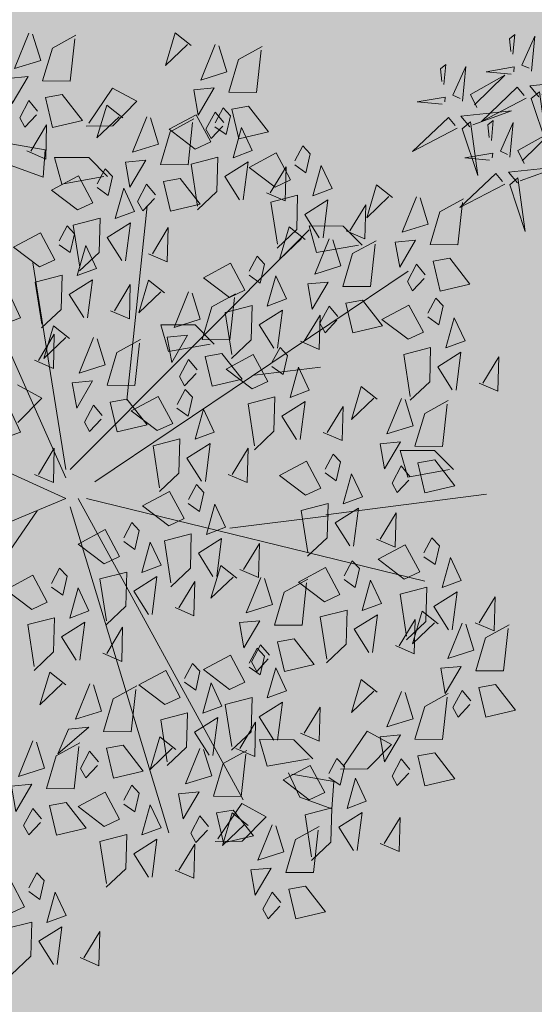
# Model space of a CAD drawing. Units: inches. Extents: x 1704 to 6393, y -157 to 1172.
# Tile 68 of 122: x 1913 to 1928, y 980 to 1010. Entities that reach past the tile are written whole.
import ezdxf

# ---------------------------------------------------------------- set-up
doc = ezdxf.new("R2010")
doc.units = ezdxf.units.IN
doc.header["$MEASUREMENT"] = 0
for name, color, linetype, lineweight in [('A-ANNO-DIMS', 7, 'Continuous', 13), ('L-shrub', 74, 'Continuous', 18), ('L-tree', 102, 'Continuous', 18)]:
    doc.layers.add(name, color=color, linetype=linetype, lineweight=lineweight)
doc.layers.add('L-HRDS-PATT', color=9, linetype='Continuous', lineweight=13, true_color=0xc5c1ba)
doc.styles.get("Standard").update_dxf_attribs({"font": 'arial.ttf'})
doc.dimstyles.get("Standard").update_dxf_attribs({"dimtxt": 6, "dimasz": 2, "dimexe": 0.18, "dimexo": 0.0625, "dimgap": 0.09, "dimtad": 0, "dimtih": 1, "dimtoh": 1, "dimdec": 1, "dimzin": 0, "dimdsep": 46, "dimlunit": 3, "dimtxsty": 'Standard', "dimblk": 'ARCHTICK', "dimcen": 0.09, "dimadec": 0, "dimazin": 0, "dimtfac": 1, "dimtdec": 1, "dimtofl": 0, "dimtmove": 0, "dimatfit": 3, "dimfxl": 1, "dimtolj": 1, "dimtzin": 0, "dimarcsym": 0})

# ---------------------------------------------------------------- blocks, each defined once
blk = doc.blocks.new('bamboo')
at = {"layer": 'L-shrub'}
for points in [[(1141.3, 824.7), (1092, 972.3), (1115.5, 803.4), (1141.3, 824.7)], [(1157.1, 823.2), (1299, 896.7), (1185.5, 788.7), (1164.2, 814.6)], [(1117, 819.1), (1145.4, 784.6), (985.2, 768.4), (1108.4, 812)], [(1291.5, 647.4), (1242.1, 795), (1265.7, 626.1), (1291.5, 647.4)], [(1095.3, 757.7), (1115.1, 716.2), (1006.1, 655.3), (1102.4, 749.1)], [(1140.9, 737.5), (1130.4, 627.4), (1170.9, 718.7), (1148, 728.8)], [(1205.3, 747.1), (1283.9, 739.5), (1195.2, 724.3), (1196.7, 740)], [(1307.2, 645.9), (1449.1, 719.5), (1335.7, 611.4), (1314.3, 637.3)], [(1073.1, 552), (1023.7, 699.6), (1047.2, 530.7), (1073.1, 552)], [(1199.3, 684.2), (1193.3, 621.3), (1210.5, 635.5), (1206.4, 675.6)], [(1088.8, 550.5), (1230.7, 624), (1117.2, 516), (1095.9, 541.8)], [(1267.2, 641.9), (1295.6, 607.4), (1135.4, 591.1), (1258.6, 634.8)], [(1245.4, 580.5), (1265.3, 538.9), (1156.3, 478), (1252.6, 571.9)], [(1355.5, 569.8), (1434.1, 562.2), (1345.4, 547), (1346.9, 562.7)], [(1048.7, 546.4), (1077.2, 511.9), (916.9, 495.7), (1040.1, 539.3)], [(1291.1, 560.2), (1280.6, 450.1), (1321.1, 541.4), (1298.2, 551.6)], [(1349.5, 506.9), (1343.5, 444), (1360.7, 458.2), (1356.6, 498.3)], [(1137.1, 474.4), (1215.7, 466.8), (1126.9, 451.6), (1128.4, 467.3)], [(1072.7, 464.7), (1062.1, 354.7), (1102.6, 446), (1079.8, 456.1)], [(1131.1, 411.5), (1125, 348.6), (1142.3, 362.8), (1138.2, 402.9)]]:
    blk.add_lwpolyline(points, dxfattribs=at)
blk = doc.blocks.new('flower shrub 3')
at = {"layer": 'L-shrub'}
for p, q in [((208.75, 44.35), (204.49, 19.45)), ((57.01, 21.38), (42.5, 35.62)), ((64.85, 35.82), (57.01, 21.38)), ((188.1, 20.61), (195.06, 39.71)), ((204.49, 19.45), (188.1, 20.61)), ((184.09, 9.47), (199.9, 13.93)), ((199.9, 13.93), (199.81, -6.4)), ((188.5, -15.39), (184.09, 9.47)), ((218.7, -20.78), (218.53, -4.82)), ((199.81, -6.4), (188.49, -17.65)), ((220.15, -6.4), (241.04, -20.58)), ((233.21, -35.02), (218.7, -20.78)), ((241.04, -20.58), (233.21, -35.02)), ((84.69, -53.7), (100.5, -49.25)), ((100.5, -49.25), (100.42, -69.58)), ((89.1, -78.57), (84.69, -53.7)), ((100.42, -69.58), (89.1, -80.83)), ((-205.99, -97.49), (-206.15, -81.53)), ((-204.54, -83.11), (-183.64, -97.29)), ((-191.47, -111.73), (-205.99, -97.49)), ((-183.64, -97.29), (-191.47, -111.73)), ((-161.53, -112.36), (-145.72, -107.91)), ((-145.72, -107.91), (-145.8, -128.24)), ((-157.12, -137.23), (-161.53, -112.36)), ((-179.93, -131.75), (-165.46, -125)), ((-166.23, -127.12), (-170.5, -152.01)), ((-145.8, -128.24), (-157.13, -139.49)), ((-186.88, -150.86), (-179.93, -131.75)), ((143.42, -141.69), (159.24, -137.24)), ((159.24, -137.24), (159.15, -157.57)), ((147.84, -166.56), (143.42, -141.69)), ((-170.5, -152.01), (-186.88, -150.86)), ((-163.07, -171.95), (-163.23, -155.98)), ((-161.62, -157.57), (-140.72, -171.75)), ((159.15, -157.57), (147.83, -168.82)), ((-148.55, -186.18), (-163.07, -171.95)), ((-140.72, -171.75), (-148.55, -186.18)), ((10.15, -195.84), (25.96, -191.38)), ((25.96, -191.38), (25.88, -211.71)), ((14.56, -220.7), (10.15, -195.84)), ((25.88, -211.71), (14.55, -222.96))]:
    blk.add_line(p, q, dxfattribs=at)
for points in [[(-2.54, 7.13), (56.31, 136.92)], [(-9.89, 24.27), (-166.82, 132.02)], [(-2.54, 7.13), (-51.58, 124.68)], [(9.72, 7.13), (124.97, 58.56)], [(-249.17, 40.85), (-237.45, 56.33), (-228.85, 40.3), (-244.9, 31.7), (-249.17, 40.85)], [(-283.1, 39.51), (-258.14, 43.35), (-254.05, 27.44), (-274.37, 27.98), (-285.36, 39.57)], [(-68.45, 27.31), (-56.74, 42.79), (-48.13, 26.76), (-64.18, 18.17), (-68.45, 27.31)], [(32.59, 45.49), (36.8, 34.09), (50.54, 40.49), (32.59, 45.49)], [(100.36, 45.49), (104.57, 34.09), (118.3, 40.49), (100.36, 45.49)], [(247.89, 29.6), (246.76, 41.7), (231.84, 39.06), (247.89, 29.6)], [(-172.27, 27.35), (-173.4, 39.44), (-188.32, 36.8), (-172.27, 27.35)], [(-147.16, 24.62), (-162.72, 19.81), (-167.54, 35.36), (-146.52, 26.78)], [(134.85, 22.8), (146.57, 38.28), (155.17, 22.25), (139.12, 13.65), (134.85, 22.8)], [(273, 26.88), (257.44, 22.07), (252.62, 37.61), (273.64, 29.04)], [(-192.8, 21.66), (-186.55, 26.86), (-196.74, 32.23), (-202.35, 29.19), (-194.97, 22.3)], [(-102.39, 25.97), (-77.43, 29.81), (-73.34, 13.9), (-93.66, 14.45), (-104.64, 26.03)], [(203.73, 30.25), (198.91, 19.1), (219.23, 18.55), (203.67, 28)], [(227.36, 23.91), (233.62, 29.12), (223.43, 34.49), (217.81, 31.44), (225.2, 24.55)], [(-235.92, 29.2), (-240.62, 22.56), (-229.39, 20), (-224.76, 24.39), (-233.67, 29.14)], [(11.72, 25.74), (6.9, 14.58), (27.22, 14.04), (11.66, 23.48)], [(14.63, 7.13), (137.23, 26.72)], [(79.49, 25.74), (74.67, 14.58), (94.99, 14.04), (79.43, 23.48)], [(100.92, 21.46), (125.88, 25.3), (129.97, 9.39), (109.65, 9.94), (98.66, 21.52)], [(-279.26, 14.57), (-265.46, 23.23), (-256.8, 9.45), (-279.32, 12.32)], [(-254.29, 18.41), (-250.08, 7.02), (-236.35, 13.42), (-254.29, 18.41)], [(-149.87, -0.46), (-174.98, 2.27), (-174.83, 18.69), (-155.34, 12.92), (-147.71, -1.1)], [(-113.13, 7.2), (-105.6, 16.74), (-125.09, 22.51), (-112.49, 9.37)], [(92.43, 4.95), (99.97, 14.48), (80.47, 20.25), (93.07, 7.11)], [(237.16, 9.25), (221.85, -2.69), (217.66, 15.02), (235.39, 19.19), (237.16, 9.25)], [(270.29, 1.8), (245.18, 4.52), (245.33, 20.95), (264.83, 15.18), (272.46, 1.16)], [(-183.01, 6.99), (-198.32, -4.95), (-202.5, 12.76), (-184.78, 16.93), (-183.01, 6.99)], [(-138.39, -6.5), (-139.52, 5.6), (-154.26, 11.88), (-138.39, -6.5)], [(-55.21, 15.67), (-59.91, 9.02), (-48.68, 6.46), (-44.04, 10.85), (-52.95, 15.61)], [(168.74, 0.24), (180.45, 15.72), (189.06, -0.31), (173.01, -8.91), (168.74, 0.24)], [(-98.54, 1.04), (-84.75, 9.69), (-76.08, -4.08), (-98.6, -1.22)], [(148.1, 11.15), (143.4, 4.51), (154.63, 1.95), (159.26, 6.34), (150.35, 11.09)], [(-7.44, 4.68), (-201.15, -54.09)], [(-113.28, -9.22), (-128.84, -14.03), (-133.66, 1.52), (-112.64, -7.06)], [(-73.58, 4.88), (-69.37, -6.52), (-55.64, -0.12), (-73.58, 4.88)], [(14.63, 4.68), (156.84, -137.36)], [(67.18, -8.75), (66.05, 3.35), (51.13, 0.7), (67.18, -8.75)], [(104.77, -3.47), (118.56, 5.18), (127.22, -8.59), (104.7, -5.73)], [(129.73, 0.37), (133.94, -11.03), (147.67, -4.63), (129.73, 0.37)], [(134.8, -1.11), (159.76, 2.73), (163.85, -13.17), (143.53, -12.63), (132.54, -1.04)], [(-275.17, -1.33), (-279.99, -12.49), (-259.66, -13.04), (-275.23, -3.59)], [(-197.21, -15.56), (-185.5, -0.08), (-176.89, -16.11), (-192.94, -24.7), (-197.21, -15.56)], [(-2.54, -0.22), (-181.53, -98.18)], [(-158.92, -12.19), (-152.66, -6.98), (-162.85, -1.61), (-168.47, -4.65), (-161.08, -11.54)], [(-2.54, -5.12), (-51.58, -205.93)], [(-41.35, -15.56), (-29.63, -0.08), (-21.02, -16.11), (-37.07, -24.7), (-41.35, -15.56)], [(46.65, -14.44), (52.9, -9.23), (42.71, -3.87), (37.1, -6.91), (44.48, -13.8)], [(92.28, -11.48), (76.73, -16.28), (71.9, -0.74), (92.92, -9.31)], [(7.27, -10.01), (132.32, -196.13)], [(181.98, -11.41), (177.28, -18.05), (188.51, -20.61), (193.15, -16.22), (184.24, -11.47)], [(223.45, -26.64), (230.99, -17.1), (211.49, -11.33), (224.09, -24.47)], [(-231.15, -16.9), (-206.18, -13.06), (-202.09, -28.97), (-222.42, -28.42), (-233.4, -16.84)], [(-149.12, -26.85), (-164.43, -38.79), (-168.62, -21.08), (-150.89, -16.91), (-149.12, -26.85)], [(-115.99, -34.3), (-141.1, -31.58), (-140.95, -15.15), (-121.45, -20.92), (-113.82, -34.94)], [(-94.45, -14.87), (-99.27, -26.03), (-78.95, -26.58), (-94.51, -17.13)], [(-75.28, -16.9), (-50.32, -13.06), (-46.23, -28.97), (-66.55, -28.42), (-77.54, -16.84)], [(89.57, -36.56), (64.47, -33.83), (64.62, -17.41), (84.11, -23.18), (91.74, -37.2)], [(138.65, -26.04), (152.44, -17.38), (161.11, -31.16), (138.59, -28.29)], [(56.44, -29.1), (41.13, -41.04), (36.95, -23.34), (54.67, -19.17), (56.44, -29.1)], [(108.86, -19.38), (104.03, -30.54), (124.36, -31.09), (108.79, -21.64)], [(163.61, -22.2), (167.82, -33.59), (181.55, -27.19), (163.61, -22.2)], [(-183.97, -27.2), (-188.67, -33.84), (-177.44, -36.4), (-172.8, -32.02), (-181.71, -27.26)], [(-28.1, -27.2), (-32.8, -33.84), (-21.57, -36.4), (-16.93, -32.02), (-25.84, -27.26)], [(55.85, -28.96), (171.09, -41.21)], [(198.2, -40.34), (197.06, -28.24), (182.15, -30.88), (198.2, -40.34)], [(-227.3, -41.83), (-213.51, -33.17), (-204.84, -46.95), (-227.36, -44.08)], [(-71.43, -41.83), (-57.64, -33.17), (-48.97, -46.95), (-71.49, -44.08)], [(37.72, -47.14), (49.43, -31.66), (58.04, -47.69), (41.99, -56.29), (37.72, -47.14)], [(223.3, -43.06), (207.75, -47.87), (202.92, -32.33), (223.94, -40.9)], [(-202.34, -37.99), (-198.13, -49.39), (-184.4, -42.99), (-202.34, -37.99)], [(-124.93, -51.66), (-113.21, -36.17), (-104.6, -52.2), (-120.65, -60.8), (-124.93, -51.66)], [(-46.47, -37.99), (-42.26, -49.39), (-28.53, -42.99), (-46.47, -37.99)], [(-18.76, -53.91), (-7.04, -38.43), (1.57, -54.46), (-14.48, -63.06), (-18.76, -53.91)], [(119.54, -51.46), (127.07, -41.92), (107.58, -36.15), (120.18, -49.29)], [(177.67, -46.03), (183.92, -40.82), (173.73, -35.45), (168.12, -38.5), (175.5, -45.39)], [(-151.53, -58.22), (-144, -48.69), (-163.49, -42.92), (-150.89, -56.06)], [(3.78, -48.48), (28.75, -44.64), (32.84, -60.55), (12.51, -60.01), (1.53, -48.42)], [(142.74, -41.95), (137.92, -53.1), (158.24, -53.65), (142.68, -44.2)], [(-158.86, -53), (-133.9, -49.16), (-129.81, -65.07), (-150.13, -64.52), (-161.12, -52.94)], [(-52.69, -55.25), (-27.73, -51.41), (-23.64, -67.32), (-43.96, -66.77), (-54.95, -55.19)], [(187.46, -60.69), (172.15, -72.63), (167.97, -54.92), (185.69, -50.76), (187.46, -60.69)], [(220.59, -68.14), (195.49, -65.42), (195.64, -48.99), (215.13, -54.76), (222.76, -68.78)], [(266.37, -67.25), (273.91, -57.71), (254.41, -51.94), (267.01, -65.08)], [(-223.21, -57.74), (-228.03, -68.89), (-207.71, -69.44), (-223.27, -59.99)], [(-67.34, -57.74), (-72.16, -68.89), (-51.84, -69.44), (-67.4, -59.99)], [(94.28, -65.16), (93.15, -53.06), (78.24, -55.7), (94.28, -65.16)], [(119.39, -67.88), (103.83, -72.69), (99.01, -57.14), (120.03, -65.72)], [(204.88, -69.71), (216.6, -54.22), (225.2, -70.25), (209.15, -78.85), (204.88, -69.71)], [(-176.79, -71.93), (-177.92, -59.83), (-192.84, -62.47), (-176.79, -71.93)], [(-151.68, -74.65), (-167.24, -79.46), (-172.06, -63.91), (-151.04, -72.49)], [(-111.68, -63.3), (-116.38, -69.94), (-105.15, -72.5), (-100.51, -68.11), (-109.42, -63.36)], [(50.96, -58.79), (46.26, -65.43), (57.49, -67.99), (62.13, -63.6), (53.22, -58.85)], [(73.75, -70.85), (80.01, -65.64), (69.82, -60.27), (64.2, -63.31), (71.59, -70.2)], [(-197.32, -77.61), (-191.07, -72.41), (-201.26, -67.04), (-206.87, -70.08), (-199.48, -76.97)], [(-155.01, -77.93), (-141.22, -69.27), (-132.55, -83.05), (-155.07, -80.18)], [(-5.51, -65.55), (-10.21, -72.2), (1.02, -74.76), (5.66, -70.37), (-3.25, -65.62)], [(7.63, -73.42), (21.42, -64.76), (30.09, -78.54), (7.57, -75.67)], [(32.59, -69.58), (36.8, -80.97), (50.54, -74.57), (32.59, -69.58)], [(170.95, -71.05), (195.91, -67.21), (200, -83.12), (179.67, -82.57), (168.69, -70.99)], [(241.12, -80.95), (239.98, -68.85), (225.07, -71.49), (241.12, -80.95)], [(-130.05, -74.09), (-125.84, -85.49), (-112.11, -79.09), (-130.05, -74.09)], [(-115.89, -90.01), (-104.17, -74.53), (-95.57, -90.56), (-111.62, -99.15), (-115.89, -90.01)], [(-48.84, -80.18), (-35.05, -71.53), (-26.38, -85.3), (-48.9, -82.44)], [(83.55, -85.51), (68.24, -97.45), (64.06, -79.74), (81.78, -75.57), (83.55, -85.51)], [(116.68, -92.96), (91.57, -90.24), (91.72, -73.81), (111.22, -79.58), (118.85, -93.6)], [(116.78, -90.01), (128.5, -74.53), (137.1, -90.56), (121.05, -99.15), (116.78, -90.01)], [(266.22, -83.67), (250.67, -88.48), (245.84, -72.94), (266.86, -81.51)], [(-154.39, -99.73), (-179.5, -97), (-179.35, -80.58), (-159.85, -86.35), (-152.23, -100.37)], [(-49.88, -94.32), (-42.35, -84.79), (-61.84, -79.02), (-49.24, -92.16)], [(-23.88, -76.34), (-19.67, -87.74), (-5.94, -81.34), (-23.88, -76.34)], [(220.59, -86.64), (226.84, -81.43), (216.65, -76.06), (211.04, -79.11), (218.42, -86)], [(218.12, -81.35), (213.42, -87.99), (224.65, -90.55), (229.29, -86.16), (220.38, -81.41)], [(-196.71, -101.09), (-189.18, -91.56), (-208.67, -85.79), (-196.07, -98.93)], [(-187.52, -92.28), (-202.84, -104.22), (-207.02, -86.51), (-189.29, -82.34), (-187.52, -92.28)], [(-149.82, -91.35), (-124.86, -87.51), (-120.77, -103.42), (-141.1, -102.87), (-152.08, -91.29)], [(82.85, -91.35), (107.81, -87.51), (111.9, -103.42), (91.58, -102.87), (80.59, -91.29)], [(174.79, -95.98), (188.58, -87.32), (197.25, -101.1), (174.73, -98.23)], [(-12.8, -148.96), (-20.16, -90.19)], [(11.72, -89.32), (6.9, -100.48), (27.22, -101.03), (11.66, -91.58)], [(62.57, -103.55), (74.28, -88.07), (82.89, -104.1), (66.84, -112.69), (62.57, -103.55)], [(199.75, -92.14), (203.97, -103.54), (217.7, -97.14), (199.75, -92.14)], [(230.38, -101.3), (215.07, -113.24), (210.89, -95.53), (228.61, -91.37), (230.38, -101.3)], [(263.51, -108.75), (238.41, -106.03), (238.56, -89.6), (258.05, -95.37), (265.68, -109.39)], [(-150.92, -93.84), (-155.74, -104.99), (-135.42, -105.54), (-150.98, -96.09)], [(-75.14, -108.02), (-76.27, -95.92), (-91.18, -98.57), (-75.14, -108.02)], [(-44.75, -96.09), (-49.57, -107.25), (-29.25, -107.8), (-44.81, -98.35)], [(-221.97, -114.79), (-223.1, -102.69), (-238.02, -105.34), (-221.97, -114.79)], [(-102.65, -101.65), (-107.35, -108.3), (-96.12, -110.86), (-91.48, -106.47), (-100.39, -101.71)], [(-95.67, -113.71), (-89.41, -108.5), (-99.6, -103.14), (-105.22, -106.18), (-97.83, -113.07)], [(-50.03, -110.75), (-65.59, -115.56), (-70.41, -100.01), (-49.39, -108.58)], [(28.63, -104.89), (53.59, -101.05), (57.68, -116.96), (37.36, -116.41), (26.37, -104.83)], [(70.56, -104.88), (75.47, -144.06)], [(130.02, -101.65), (125.33, -108.3), (136.56, -110.86), (141.19, -106.47), (132.28, -101.71)], [(182.29, -117.08), (194.01, -101.6), (202.61, -117.63), (186.56, -126.23), (182.29, -117.08)], [(-242.5, -120.48), (-236.24, -115.27), (-246.44, -109.9), (-252.05, -112.95), (-244.66, -119.84)], [(-196.86, -117.52), (-212.42, -122.32), (-217.24, -106.78), (-196.22, -115.35)], [(-145.98, -116.28), (-132.19, -107.63), (-123.52, -121.4), (-146.04, -118.54)], [(86.69, -116.28), (100.49, -107.63), (109.15, -121.4), (86.63, -118.54)], [(-121.02, -112.44), (-116.8, -123.84), (-103.07, -117.44), (-121.02, -112.44)], [(-52.74, -135.83), (-77.85, -133.1), (-77.7, -116.68), (-58.2, -122.45), (-50.57, -136.47)], [(75.81, -115.19), (71.11, -121.83), (82.34, -124.39), (86.98, -120.01), (78.07, -115.25)], [(111.65, -112.44), (115.87, -123.84), (129.6, -117.44), (111.65, -112.44)], [(148.36, -118.43), (173.32, -114.59), (177.41, -130.49), (157.08, -129.95), (146.1, -118.36)], [(178.88, -111.89), (174.06, -123.04), (194.39, -123.59), (178.82, -114.14)], [(-181.4, -137.39), (-169.68, -121.91), (-161.08, -137.94), (-177.13, -146.53), (-181.4, -137.39)], [(-85.87, -128.38), (-101.18, -140.31), (-105.37, -122.61), (-87.64, -118.44), (-85.87, -128.38)], [(-0.69, -135.13), (11.03, -119.65), (19.64, -135.68), (3.59, -144.28), (-0.69, -135.13)], [(32.48, -129.82), (46.27, -121.16), (54.94, -134.94), (32.42, -132.07)], [(151.17, -134.93), (158.7, -125.4), (139.2, -119.63), (151.81, -132.77)], [(-232.7, -135.14), (-248.01, -147.08), (-252.2, -129.38), (-234.47, -125.21), (-232.7, -135.14)], [(-199.57, -142.6), (-224.68, -139.87), (-224.53, -123.45), (-205.03, -129.21), (-197.4, -143.24)], [(57.44, -125.98), (61.65, -137.38), (75.38, -130.98), (57.44, -125.98)], [(-141.89, -132.19), (-146.71, -143.35), (-126.38, -143.9), (-141.95, -134.45)], [(-63.94, -146.41), (-52.22, -130.93), (-43.61, -146.96), (-59.66, -155.56), (-63.94, -146.41)], [(-34.62, -136.47), (-9.66, -132.63), (-5.57, -148.54), (-25.89, -148), (-36.88, -136.41)], [(90.78, -132.19), (85.96, -143.35), (106.29, -143.9), (90.72, -134.45)], [(195.53, -128.73), (190.83, -135.37), (202.06, -137.93), (206.7, -133.54), (197.79, -128.79)], [(-215.33, -138.73), (-190.37, -134.89), (-186.28, -150.8), (-206.61, -150.25), (-217.59, -138.67)], [(125.91, -148.63), (124.78, -136.54), (109.86, -139.18), (125.91, -148.63)], [(152.2, -143.36), (166, -134.7), (174.66, -148.48), (152.14, -145.61)], [(177.16, -139.52), (181.38, -150.91), (195.11, -144.51), (177.16, -139.52)], [(-97.87, -147.76), (-72.91, -143.92), (-68.82, -159.82), (-89.14, -159.28), (-100.13, -147.69)], [(36.57, -145.73), (31.75, -156.88), (52.07, -157.43), (36.51, -147.98)], [(105.38, -154.32), (111.63, -149.12), (101.44, -143.75), (95.83, -146.79), (103.21, -153.68)], [(151.02, -151.36), (135.46, -156.17), (130.64, -140.62), (151.66, -149.2)], [(-168.16, -149.03), (-172.86, -155.68), (-161.63, -158.24), (-156.99, -153.85), (-165.9, -149.09)], [(-12.34, -147.15), (-0.08, -242.66)], [(12.56, -146.78), (7.86, -153.42), (19.09, -155.98), (23.73, -151.59), (14.82, -146.84)], [(-211.49, -163.66), (-197.69, -155.01), (-189.03, -168.78), (-211.55, -165.92)], [(-30.77, -161.41), (-16.98, -152.75), (-8.31, -166.53), (-30.83, -163.66)], [(-5.81, -157.57), (-1.6, -168.96), (12.13, -162.56), (-5.81, -157.57)], [(148.31, -176.44), (123.2, -173.71), (123.35, -157.29), (142.84, -163.06), (150.47, -177.08)], [(-186.53, -159.82), (-182.31, -171.22), (-168.58, -164.82), (-186.53, -159.82)], [(-117.65, -177.8), (-110.11, -168.26), (-129.61, -162.5), (-117.01, -175.64)], [(-50.69, -158.06), (-55.39, -164.7), (-44.16, -167.26), (-39.52, -162.87), (-48.43, -158.12)], [(56.29, -177.8), (63.82, -168.26), (44.33, -162.5), (56.93, -175.64)], [(115.18, -168.99), (99.86, -180.93), (95.68, -163.22), (113.4, -159.05), (115.18, -168.99)], [(156.29, -159.27), (151.47, -170.42), (171.8, -170.97), (156.23, -161.52)], [(-94.02, -172.69), (-80.23, -164.03), (-71.56, -177.81), (-94.08, -174.94)], [(-69.06, -168.85), (-64.85, -180.24), (-51.12, -173.84), (-69.06, -168.85)], [(176.01, -186.82), (183.55, -177.29), (164.05, -171.52), (176.66, -184.66)], [(-207.4, -179.57), (-212.22, -190.73), (-191.89, -191.27), (-207.46, -181.83)], [(-142.9, -191.5), (-144.04, -179.4), (-158.95, -182.05), (-142.9, -191.5)], [(-50.38, -193.79), (-38.67, -178.31), (-30.06, -194.34), (-46.11, -202.94), (-50.38, -193.79)], [(-26.68, -177.31), (-31.5, -188.47), (-11.18, -189.02), (-26.74, -179.57)], [(31.03, -191.5), (29.9, -179.4), (14.99, -182.05), (31.03, -191.5)], [(91.93, -196.05), (103.65, -180.57), (112.25, -196.6), (96.2, -205.19), (91.93, -196.05)], [(-163.43, -197.19), (-157.18, -191.98), (-167.37, -186.61), (-172.98, -189.66), (-165.6, -196.55)], [(-117.8, -194.23), (-133.35, -199.03), (-138.18, -183.49), (-117.16, -192.06)], [(10.5, -197.19), (16.76, -191.98), (6.57, -186.61), (0.95, -189.66), (8.34, -196.55)], [(56.14, -194.23), (40.58, -199.03), (35.76, -183.49), (56.78, -192.06)], [(-89.93, -188.6), (-94.75, -199.75), (-74.43, -200.3), (-89.99, -190.85)], [(-84.31, -195.13), (-59.35, -191.29), (-55.26, -207.2), (-75.59, -206.66), (-86.57, -195.07)], [(150.76, -200.53), (149.63, -188.43), (134.71, -191.07), (150.76, -200.53)], [(175.87, -203.25), (160.31, -208.06), (155.49, -192.51), (176.51, -201.09)], [(-76.99, -213.9), (-69.45, -204.36), (-88.95, -198.59), (-76.35, -211.73)], [(58, -197.39), (82.96, -193.55), (87.05, -209.46), (66.73, -208.91), (55.74, -197.33)], [(130.23, -206.21), (136.48, -201.01), (126.29, -195.64), (120.68, -198.68), (128.06, -205.57)], [(-153.64, -211.85), (-168.95, -223.79), (-173.13, -206.08), (-155.41, -201.92), (-153.64, -211.85)], [(-120.51, -219.31), (-145.61, -216.58), (-145.47, -200.15), (-125.97, -205.92), (-118.34, -219.95)], [(20.3, -211.85), (4.99, -223.79), (0.8, -206.08), (18.53, -201.92), (20.3, -211.85)], [(53.43, -219.31), (28.32, -216.58), (28.47, -200.15), (47.97, -205.92), (55.6, -219.95)], [(-37.14, -205.44), (-41.84, -212.08), (-30.61, -214.64), (-25.97, -210.25), (-34.88, -205.5)], [(105.18, -207.69), (100.48, -214.34), (111.71, -216.9), (116.34, -212.51), (107.43, -207.75)], [(173.16, -228.33), (148.05, -225.61), (148.2, -209.18), (167.69, -214.95), (175.32, -228.97)], [(-102.24, -227.6), (-103.37, -215.5), (-118.29, -218.14), (-102.24, -227.6)], [(-80.47, -220.07), (-66.68, -211.41), (-58.01, -225.19), (-80.53, -222.32)], [(-55.51, -216.23), (-51.3, -227.62), (-37.56, -221.22), (-55.51, -216.23)], [(61.85, -222.32), (75.64, -213.67), (84.3, -227.44), (61.78, -224.58)], [(140.02, -220.88), (124.71, -232.82), (120.53, -215.11), (138.25, -210.94), (140.02, -220.88)], [(-77.14, -230.32), (-92.69, -235.13), (-97.52, -219.59), (-76.5, -228.16)], [(86.81, -218.48), (91.02, -229.88), (104.75, -223.48), (86.81, -218.48)], [(-122.77, -233.29), (-116.52, -228.08), (-126.71, -222.71), (-132.32, -225.76), (-124.94, -232.65)], [(-112.98, -247.95), (-128.29, -259.89), (-132.47, -242.18), (-114.75, -238.02), (-112.98, -247.95)], [(-79.85, -255.4), (-104.95, -252.68), (-104.8, -236.25), (-85.31, -242.02), (-77.68, -256.04)], [(-76.38, -235.97), (-81.2, -247.13), (-60.88, -247.68), (-76.44, -238.23)], [(65.94, -238.23), (61.11, -249.39), (81.44, -249.93), (65.87, -240.49)]]:
    blk.add_lwpolyline(points, dxfattribs=at)
blk = doc.blocks.new('_ArchTick')
at = {"color": 0, "linetype": 'ByBlock', "const_width": 0.15}
blk.add_lwpolyline([(-0.5, -0.5), (0.5, 0.5)], dxfattribs=at)
blk = doc.blocks.new('*D94')
at = {"layer": 'A-ANNO-DIMS', "color": 0, "lineweight": -2, "transparency": 16777216}
for p, q in [((1898.349, 895.275), (1898.349, 1105.287)), ((2073.349, 895.275), (2073.349, 1105.287)), ((1898.349, 1105.107), (1979.39, 1105.107)), ((2073.349, 1105.107), (1992.307, 1105.107))]:
    blk.add_line(p, q, dxfattribs=at)
at = {"layer": 'Defpoints', "color": 0, "lineweight": -3, "transparency": 16777216}
for p in [(2073.349, 1105.107), (1898.349, 895.213), (2073.349, 895.213)]:
    blk.add_point(p, dxfattribs=at)
at = {"layer": 'A-ANNO-DIMS', "color": 0, "lineweight": -2, "transparency": 16777216, "xscale": 2, "yscale": 2, "zscale": 2, "rotation": 180}
blk.add_blockref('_ArchTick', (1898.349, 1105.107), dxfattribs=at)
at = {"layer": 'A-ANNO-DIMS', "color": 0, "lineweight": -2, "transparency": 16777216, "xscale": 2, "yscale": 2, "zscale": 2}
blk.add_blockref('_ArchTick', (2073.349, 1105.107), dxfattribs=at)
at = {"layer": 'A-ANNO-DIMS', "color": 0, "transparency": 16777216, "insert": (1985.849, 1105.107), "char_height": 6, "attachment_point": 5}
blk.add_mtext('\\A1;175', dxfattribs=at)

msp = doc.modelspace()

# ---------------------------------------------------------------- hatches: boundary and pattern name
at = {"layer": 'L-HRDS-PATT', "transparency": 33554643}
h = msp.add_hatch(color=256, dxfattribs=at)
h.dxf.hatch_style = 1
h.paths.add_polyline_path([(2065.589, 1033.213), (1898.349, 1033.213), (1898.349, 895.213), (2065.589, 895.213)])

# ---------------------------------------------------------------- block references
at = {"layer": 'L-shrub', "xscale": 0.0510581485411622, "yscale": 0.0510581485411622, "zscale": 0.0510581485411622, "rotation": 89.99999999999996}
msp.add_blockref('flower shrub 3', (1914.61, 995.518), dxfattribs=at)
at = {"layer": 'L-tree', "xscale": 0.0095734028514679, "yscale": 0.0095734028514679, "zscale": 0.0095734028514679, "rotation": 180}
msp.add_blockref('bamboo', (1938.628, 1012.792), dxfattribs=at)

# ---------------------------------------------------------------- dimensions: what is measured, and where the dimension line sits
at = {"layer": 'A-ANNO-DIMS'}
dim = msp.add_linear_dim(base=(2073.349, 1105.107), p1=(1898.349, 895.213), p2=(2073.349, 895.213), dimstyle='Standard', override={"dimdec": 0, "dimlfac": 1, "dimrnd": 0, "dimzin": 0, "dimdsep": 46, "dimlunit": 2}, dxfattribs=at)
dim.commit()
dim.dimension.update_dxf_attribs({"geometry": '*D94', "text_midpoint": (1985.849, 1105.107)})

doc.saveas('drawing.dxf')
